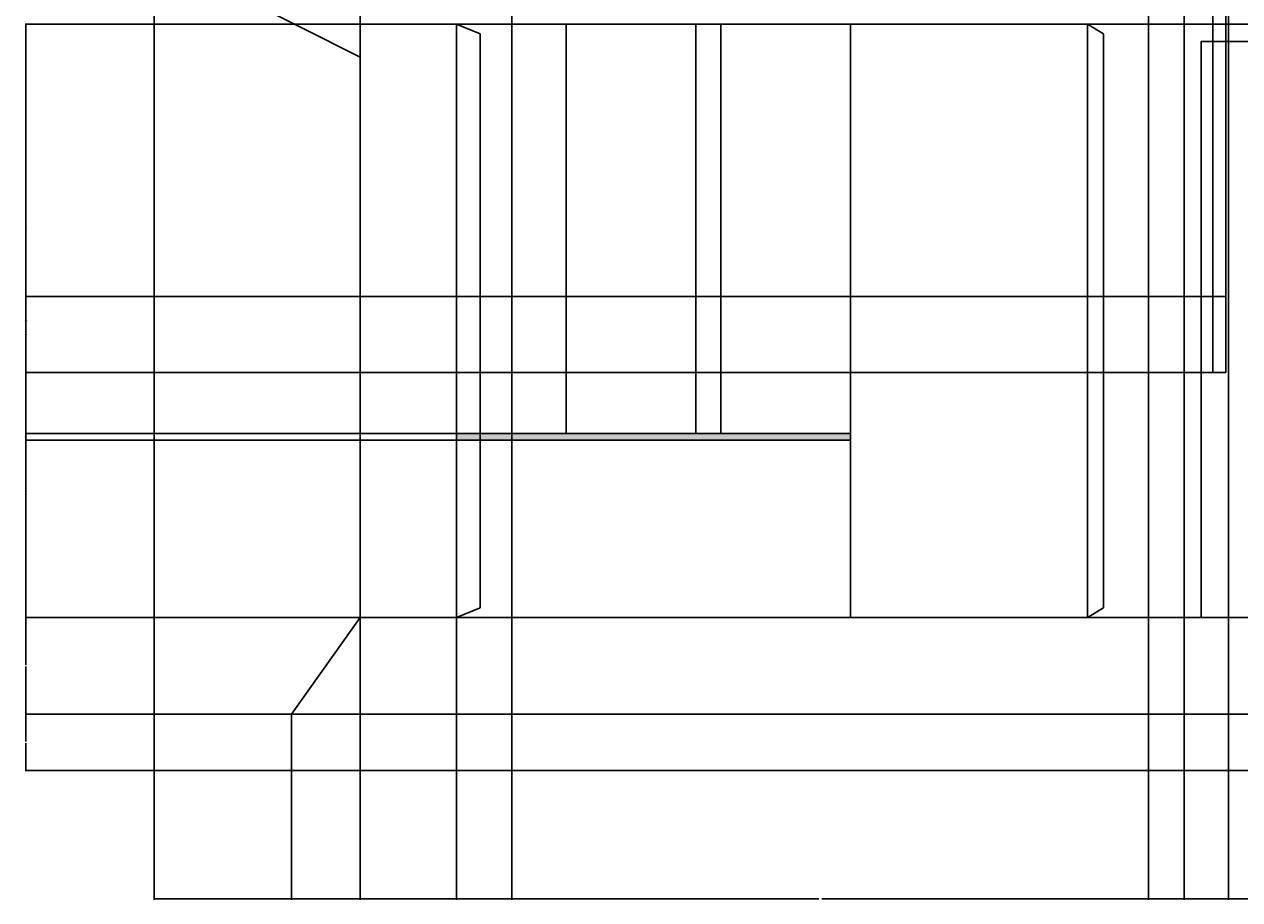
# Model space of a CAD drawing. Units: millimetres. Extents: x 171 to 1599, y 973 to 1509.
# Tile 2 of 7: x 951 to 1235, y 973 to 1178. Entities that reach past the tile are written whole.
import ezdxf

# ---------------------------------------------------------------- set-up
doc = ezdxf.new("R2010")
doc.units = ezdxf.units.MM
for name, color, linetype, lineweight in [('A-ANNO-DIMS', 2, 'Continuous', 18), ('A-ELEV', 7, 'Continuous', 25), ('A-ELEV-FILL', 252, 'Continuous', 13)]:
    doc.layers.add(name, color=color, linetype=linetype, lineweight=lineweight)
doc.styles.get("Standard").update_dxf_attribs({"font": 'arial.ttf'})
doc.dimstyles.get("Standard").update_dxf_attribs({"dimtxt": 0.18, "dimasz": 0.18, "dimexe": 0.18, "dimexo": 0.0625, "dimgap": 0.09, "dimtad": 0, "dimtih": 1, "dimtoh": 1, "dimdec": 1, "dimzin": 0, "dimdsep": 46, "dimlunit": 3, "dimtxsty": 'Standard', "dimcen": 0.09, "dimadec": 0, "dimazin": 0, "dimtfac": 1, "dimtdec": 1, "dimtofl": 0, "dimtmove": 0, "dimatfit": 3, "dimfxl": 1, "dimtolj": 1, "dimtzin": 0, "dimarcsym": 0})

# ---------------------------------------------------------------- blocks, each defined once
blk = doc.blocks.new('*D2')
at = {"layer": 'A-ANNO-DIMS', "color": 0, "lineweight": -2, "transparency": 16777216}
for p, q in [((1043.70287, 1478.130098), (1599.212656, 1478.130098)), ((1599.032656, 1477.950098), (1599.032656, 1240.959874)), ((1599.032656, 1003.60965), (1599.032656, 1240.599874)), ((1348.449149, 1003.42965), (1599.212656, 1003.42965))]:
    blk.add_line(p, q, dxfattribs=at)
at = {"layer": 'A-ANNO-DIMS', "color": 0, "transparency": 16777216}
for points in [[(1599.002656, 1477.950098), (1599.062656, 1477.950098), (1599.032656, 1478.130098)], [(1599.002656, 1003.60965), (1599.062656, 1003.60965), (1599.032656, 1003.42965)]]:
    blk.add_solid(points, dxfattribs=at)
at = {"layer": 'Defpoints', "color": 0, "transparency": 16777216}
for p in [(1043.64037, 1478.130098), (1599.032656, 1478.130098), (1348.386649, 1003.42965)]:
    blk.add_point(p, dxfattribs=at)
at = {"layer": 'A-ANNO-DIMS', "color": 0, "transparency": 16777216, "insert": (1599.032656, 1240.779874), "char_height": 0.18, "attachment_point": 5}
blk.add_mtext('\\A1;474.7', dxfattribs=at)
blk = doc.blocks.new('*D3')
at = {"layer": 'A-ANNO-DIMS', "color": 0, "lineweight": -2, "transparency": 16777216}
for p, q in [((1029.07, 1039.19), (1029.07, 973.25)), ((1013.06, 1003.37), (1013.06, 973.25)), ((1013.24, 973.43), (1020.69, 973.43)), ((1028.89, 973.43), (1021.43, 973.43))]:
    blk.add_line(p, q, dxfattribs=at)
at = {"layer": 'A-ANNO-DIMS', "color": 0, "transparency": 16777216}
for points in [[(1013.24, 973.46), (1013.24, 973.4), (1013.06, 973.43)], [(1028.89, 973.46), (1028.89, 973.4), (1029.07, 973.43)]]:
    blk.add_solid(points, dxfattribs=at)
at = {"layer": 'Defpoints', "color": 0, "transparency": 16777216}
for p in [(1029.07, 1039.25), (1013.06, 1003.43), (1029.07, 973.43)]:
    blk.add_point(p, dxfattribs=at)
at = {"layer": 'A-ANNO-DIMS', "color": 0, "transparency": 16777216, "insert": (1021.06, 973.43), "char_height": 0.18, "attachment_point": 5}
blk.add_mtext('\\A1;16.01', dxfattribs=at)
blk = doc.blocks.new('*D4')
at = {"layer": 'A-ANNO-DIMS', "color": 0, "lineweight": -2, "transparency": 16777216}
for p, q in [((1029.07, 1039.19), (1029.07, 973.25)), ((1051.62, 1039.19), (1051.62, 973.25)), ((1029.25, 973.43), (1039.88, 973.43)), ((1051.44, 973.43), (1040.81, 973.43))]:
    blk.add_line(p, q, dxfattribs=at)
at = {"layer": 'A-ANNO-DIMS', "color": 0, "transparency": 16777216}
for points in [[(1029.25, 973.46), (1029.25, 973.4), (1029.07, 973.43)], [(1051.44, 973.46), (1051.44, 973.4), (1051.62, 973.43)]]:
    blk.add_solid(points, dxfattribs=at)
at = {"layer": 'Defpoints', "color": 0, "transparency": 16777216}
for p in [(1029.07, 1039.25), (1051.62, 1039.25), (1051.62, 973.43)]:
    blk.add_point(p, dxfattribs=at)
at = {"layer": 'A-ANNO-DIMS', "color": 0, "transparency": 16777216, "insert": (1040.34, 973.43), "char_height": 0.18, "attachment_point": 5}
blk.add_mtext('\\A1;22.556', dxfattribs=at)
blk = doc.blocks.new('*D5')
at = {"layer": 'A-ANNO-DIMS', "color": 0, "lineweight": -2, "transparency": 16777216}
for p, q in [((1051.62, 1039.19), (1051.62, 973.25)), ((1221.72, 1039.19), (1221.72, 973.25)), ((1051.8, 973.43), (1136.3, 973.43)), ((1221.54, 973.43), (1137.04, 973.43))]:
    blk.add_line(p, q, dxfattribs=at)
at = {"layer": 'A-ANNO-DIMS', "color": 0, "transparency": 16777216}
for points in [[(1051.8, 973.46), (1051.8, 973.4), (1051.62, 973.43)], [(1221.54, 973.46), (1221.54, 973.4), (1221.72, 973.43)]]:
    blk.add_solid(points, dxfattribs=at)
at = {"layer": 'Defpoints', "color": 0, "transparency": 16777216}
for p in [(1051.62, 1039.25), (1221.72, 1039.25), (1221.72, 973.43)]:
    blk.add_point(p, dxfattribs=at)
at = {"layer": 'A-ANNO-DIMS', "color": 0, "transparency": 16777216, "insert": (1136.67, 973.43), "char_height": 0.18, "attachment_point": 5}
blk.add_mtext('\\A1;170.1', dxfattribs=at)
blk = doc.blocks.new('*D6')
at = {"layer": 'A-ANNO-DIMS', "color": 0, "lineweight": -2, "transparency": 16777216}
for p, q in [((1221.72, 1039.19), (1221.72, 973.25)), ((1298.24, 1039.19), (1298.24, 973.25)), ((1221.9, 973.43), (1259.59, 973.43)), ((1298.06, 973.43), (1260.37, 973.43))]:
    blk.add_line(p, q, dxfattribs=at)
at = {"layer": 'A-ANNO-DIMS', "color": 0, "transparency": 16777216}
for points in [[(1221.9, 973.46), (1221.9, 973.4), (1221.72, 973.43)], [(1298.06, 973.46), (1298.06, 973.4), (1298.24, 973.43)]]:
    blk.add_solid(points, dxfattribs=at)
at = {"layer": 'Defpoints', "color": 0, "transparency": 16777216}
for p in [(1221.72, 1039.25), (1298.24, 1039.25), (1298.24, 973.43)]:
    blk.add_point(p, dxfattribs=at)
at = {"layer": 'A-ANNO-DIMS', "color": 0, "transparency": 16777216, "insert": (1259.98, 973.43), "char_height": 0.18, "attachment_point": 5}
blk.add_mtext('\\A1;76.52', dxfattribs=at)
blk = doc.blocks.new('*D11')
at = {"layer": 'A-ANNO-DIMS', "color": 0, "lineweight": -2, "transparency": 16777216}
for p, q in [((1012.99, 1016.64), (950.75, 1016.64)), ((950.93, 1016.46), (950.93, 1010.22)), ((950.93, 1003.61), (950.93, 1009.85)), ((1012.99, 1003.43), (950.75, 1003.43))]:
    blk.add_line(p, q, dxfattribs=at)
at = {"layer": 'A-ANNO-DIMS', "color": 0, "transparency": 16777216}
for points in [[(950.9, 1016.46), (950.96, 1016.46), (950.93, 1016.64)], [(950.9, 1003.61), (950.96, 1003.61), (950.93, 1003.43)]]:
    blk.add_solid(points, dxfattribs=at)
at = {"layer": 'Defpoints', "color": 0, "transparency": 16777216}
for p in [(950.93, 1016.64), (1013.06, 1016.64), (1013.06, 1003.43)]:
    blk.add_point(p, dxfattribs=at)
at = {"layer": 'A-ANNO-DIMS', "color": 0, "transparency": 16777216, "insert": (950.93, 1010.03), "char_height": 0.18, "attachment_point": 5}
blk.add_mtext('\\A1;13.21', dxfattribs=at)
blk = doc.blocks.new('*D12')
at = {"layer": 'A-ANNO-DIMS', "color": 0, "lineweight": -2, "transparency": 16777216}
for p, q in [((1029, 1039.25), (950.75, 1039.25)), ((950.93, 1039.07), (950.93, 1028.13)), ((950.93, 1016.82), (950.93, 1027.76)), ((1012.99, 1016.64), (950.75, 1016.64))]:
    blk.add_line(p, q, dxfattribs=at)
at = {"layer": 'A-ANNO-DIMS', "color": 0, "transparency": 16777216}
for points in [[(950.9, 1039.07), (950.96, 1039.07), (950.93, 1039.25)], [(950.9, 1016.82), (950.96, 1016.82), (950.93, 1016.64)]]:
    blk.add_solid(points, dxfattribs=at)
at = {"layer": 'Defpoints', "color": 0, "transparency": 16777216}
for p in [(950.93, 1039.25), (1029.07, 1039.25), (1013.06, 1016.64)]:
    blk.add_point(p, dxfattribs=at)
at = {"layer": 'A-ANNO-DIMS', "color": 0, "transparency": 16777216, "insert": (950.93, 1027.94), "char_height": 0.18, "attachment_point": 5}
blk.add_mtext('\\A1;22.61', dxfattribs=at)
blk = doc.blocks.new('*D13')
at = {"layer": 'A-ANNO-DIMS', "color": 0, "lineweight": -2, "transparency": 16777216}
for p, q in [((1029, 1177.87), (950.75, 1177.87)), ((950.93, 1177.69), (950.93, 1108.74)), ((950.93, 1039.43), (950.93, 1108.38)), ((1029, 1039.25), (950.75, 1039.25))]:
    blk.add_line(p, q, dxfattribs=at)
at = {"layer": 'A-ANNO-DIMS', "color": 0, "transparency": 16777216}
for points in [[(950.9, 1177.69), (950.96, 1177.69), (950.93, 1177.87)], [(950.9, 1039.43), (950.96, 1039.43), (950.93, 1039.25)]]:
    blk.add_solid(points, dxfattribs=at)
at = {"layer": 'Defpoints', "color": 0, "transparency": 16777216}
for p in [(950.93, 1177.87), (1029.07, 1177.87), (1029.07, 1039.25)]:
    blk.add_point(p, dxfattribs=at)
at = {"layer": 'A-ANNO-DIMS', "color": 0, "transparency": 16777216, "insert": (950.93, 1108.56), "char_height": 0.18, "attachment_point": 5}
blk.add_mtext('\\A1;138.62', dxfattribs=at)
blk = doc.blocks.new('*D52')
at = {"layer": 'A-ANNO-DIMS', "color": 0, "lineweight": -2, "transparency": 16777216}
for p, q in [((1064.5, 1203.73), (1064.5, 973.25)), ((980.93, 1194.43), (980.93, 973.25)), ((981.11, 973.43), (1022.32, 973.43)), ((1064.32, 973.43), (1023.11, 973.43))]:
    blk.add_line(p, q, dxfattribs=at)
at = {"layer": 'A-ANNO-DIMS', "color": 0, "transparency": 16777216}
for points in [[(981.11, 973.46), (981.11, 973.4), (980.93, 973.43)], [(1064.32, 973.46), (1064.32, 973.4), (1064.5, 973.43)]]:
    blk.add_solid(points, dxfattribs=at)
at = {"layer": 'Defpoints', "color": 0, "transparency": 16777216}
for p in [(1064.5, 1203.79), (980.93, 1194.49), (1064.5, 973.43)]:
    blk.add_point(p, dxfattribs=at)
at = {"layer": 'A-ANNO-DIMS', "color": 0, "transparency": 16777216, "insert": (1022.72, 973.43), "char_height": 0.18, "attachment_point": 5}
blk.add_mtext('\\A1;83.57', dxfattribs=at)
blk = doc.blocks.new('*D53')
at = {"layer": 'A-ANNO-DIMS', "color": 0, "lineweight": -2, "transparency": 16777216}
for p, q in [((1213.35, 1203.73), (1213.35, 973.25)), ((1232.1, 1203.73), (1232.1, 973.25)), ((1213.53, 973.43), (1222.34, 973.43)), ((1231.92, 973.43), (1223.11, 973.43))]:
    blk.add_line(p, q, dxfattribs=at)
at = {"layer": 'A-ANNO-DIMS', "color": 0, "transparency": 16777216}
for points in [[(1213.53, 973.46), (1213.53, 973.4), (1213.35, 973.43)], [(1231.92, 973.46), (1231.92, 973.4), (1232.1, 973.43)]]:
    blk.add_solid(points, dxfattribs=at)
at = {"layer": 'Defpoints', "color": 0, "transparency": 16777216}
for p in [(1213.35, 1203.79), (1232.1, 1203.79), (1232.1, 973.43)]:
    blk.add_point(p, dxfattribs=at)
at = {"layer": 'A-ANNO-DIMS', "color": 0, "transparency": 16777216, "insert": (1222.72, 973.43), "char_height": 0.18, "attachment_point": 5}
blk.add_mtext('\\A1;18.75', dxfattribs=at)
blk = doc.blocks.new('*D54')
at = {"layer": 'A-ANNO-DIMS', "color": 0, "lineweight": -2, "transparency": 16777216}
for p, q in [((1232.1, 1203.73), (1232.1, 973.25)), ((1320.32, 1192.2), (1320.32, 973.25)), ((1232.28, 973.43), (1275.82, 973.43)), ((1320.14, 973.43), (1276.6, 973.43))]:
    blk.add_line(p, q, dxfattribs=at)
at = {"layer": 'A-ANNO-DIMS', "color": 0, "transparency": 16777216}
for points in [[(1232.28, 973.46), (1232.28, 973.4), (1232.1, 973.43)], [(1320.14, 973.46), (1320.14, 973.4), (1320.32, 973.43)]]:
    blk.add_solid(points, dxfattribs=at)
at = {"layer": 'Defpoints', "color": 0, "transparency": 16777216}
for p in [(1232.1, 1203.79), (1320.32, 1192.27), (1320.32, 973.43)]:
    blk.add_point(p, dxfattribs=at)
at = {"layer": 'A-ANNO-DIMS', "color": 0, "transparency": 16777216, "insert": (1276.21, 973.43), "char_height": 0.18, "attachment_point": 5}
blk.add_mtext('\\A1;88.22', dxfattribs=at)
blk = doc.blocks.new('*D71')
at = {"layer": 'A-ANNO-DIMS', "color": 0, "lineweight": -2, "transparency": 16777216}
for p, q in [((1221.72, 1177.93), (1221.72, 1508.31)), ((1221.9, 1508.13), (1224.73, 1508.13)), ((1228.22, 1508.13), (1225.38, 1508.13)), ((1228.4, 1114.32), (1228.4, 1508.31))]:
    blk.add_line(p, q, dxfattribs=at)
at = {"layer": 'A-ANNO-DIMS', "color": 0, "transparency": 16777216}
for points in [[(1221.9, 1508.16), (1221.9, 1508.1), (1221.72, 1508.13)], [(1228.22, 1508.16), (1228.22, 1508.1), (1228.4, 1508.13)]]:
    blk.add_solid(points, dxfattribs=at)
at = {"layer": 'Defpoints', "color": 0, "transparency": 16777216}
for p in [(1228.4, 1508.13), (1221.72, 1177.87), (1228.4, 1114.25)]:
    blk.add_point(p, dxfattribs=at)
at = {"layer": 'A-ANNO-DIMS', "color": 0, "transparency": 16777216, "insert": (1225.06, 1508.13), "char_height": 0.18, "attachment_point": 5}
blk.add_mtext('\\A1;6.68', dxfattribs=at)
blk = doc.blocks.new('*D72')
at = {"layer": 'A-ANNO-DIMS', "color": 0, "lineweight": -2, "transparency": 16777216}
for p, q in [((1228.4, 1114.32), (1228.4, 1508.31)), ((1228.58, 1508.13), (1229.61, 1508.13)), ((1231.28, 1508.13), (1230.25, 1508.13)), ((1231.46, 1114.32), (1231.46, 1508.31))]:
    blk.add_line(p, q, dxfattribs=at)
at = {"layer": 'A-ANNO-DIMS', "color": 0, "transparency": 16777216}
for points in [[(1228.58, 1508.16), (1228.58, 1508.1), (1228.4, 1508.13)], [(1231.28, 1508.16), (1231.28, 1508.1), (1231.46, 1508.13)]]:
    blk.add_solid(points, dxfattribs=at)
at = {"layer": 'Defpoints', "color": 0, "transparency": 16777216}
for p in [(1231.46, 1508.13), (1228.4, 1114.25), (1231.46, 1114.25)]:
    blk.add_point(p, dxfattribs=at)
at = {"layer": 'A-ANNO-DIMS', "color": 0, "transparency": 16777216, "insert": (1229.93, 1508.13), "char_height": 0.18, "attachment_point": 5}
blk.add_mtext('\\A1;3.06', dxfattribs=at)
blk = doc.blocks.new('*D73')
at = {"layer": 'A-ANNO-DIMS', "color": 0, "lineweight": -2, "transparency": 16777216}
for p, q in [((1231.46, 1114.32), (1231.46, 1508.31)), ((1231.64, 1508.13), (1234.06, 1508.13)), ((1237.13, 1508.13), (1234.71, 1508.13)), ((1237.31, 1162.35), (1237.31, 1508.31))]:
    blk.add_line(p, q, dxfattribs=at)
at = {"layer": 'A-ANNO-DIMS', "color": 0, "transparency": 16777216}
for points in [[(1231.64, 1508.16), (1231.64, 1508.1), (1231.46, 1508.13)], [(1237.13, 1508.16), (1237.13, 1508.1), (1237.31, 1508.13)]]:
    blk.add_solid(points, dxfattribs=at)
at = {"layer": 'Defpoints', "color": 0, "transparency": 16777216}
for p in [(1237.31, 1508.13), (1237.31, 1162.29), (1231.46, 1114.25)]:
    blk.add_point(p, dxfattribs=at)
at = {"layer": 'A-ANNO-DIMS', "color": 0, "transparency": 16777216, "insert": (1234.38, 1508.13), "char_height": 0.18, "attachment_point": 5}
blk.add_mtext('\\A1;5.85', dxfattribs=at)
blk = doc.blocks.new('*D81')
at = {"layer": 'A-ANNO-DIMS', "color": 0, "lineweight": -2, "transparency": 16777216}
for p, q in [((1143.64, 1080.67), (950.75, 1080.67)), ((950.93, 1080.49), (950.93, 1060.14)), ((950.93, 1039.43), (950.93, 1059.78)), ((1143.64, 1039.25), (950.75, 1039.25))]:
    blk.add_line(p, q, dxfattribs=at)
at = {"layer": 'A-ANNO-DIMS', "color": 0, "transparency": 16777216}
for points in [[(950.9, 1080.49), (950.96, 1080.49), (950.93, 1080.67)], [(950.9, 1039.43), (950.96, 1039.43), (950.93, 1039.25)]]:
    blk.add_solid(points, dxfattribs=at)
at = {"layer": 'Defpoints', "color": 0, "transparency": 16777216}
for p in [(950.93, 1080.67), (1143.7, 1080.67), (1143.7, 1039.25)]:
    blk.add_point(p, dxfattribs=at)
at = {"layer": 'A-ANNO-DIMS', "color": 0, "transparency": 16777216, "insert": (950.93, 1059.96), "char_height": 0.18, "attachment_point": 5}
blk.add_mtext('\\A1;41.42', dxfattribs=at)
blk = doc.blocks.new('*D82')
at = {"layer": 'A-ANNO-DIMS', "color": 0, "lineweight": -2, "transparency": 16777216}
for p, q in [((1143.64, 1082.23), (950.75, 1082.23)), ((1143.64, 1080.67), (950.75, 1080.67)), ((950.93, 1082.05), (950.93, 1081.63)), ((950.93, 1080.85), (950.93, 1081.27))]:
    blk.add_line(p, q, dxfattribs=at)
at = {"layer": 'A-ANNO-DIMS', "color": 0, "transparency": 16777216}
for points in [[(950.9, 1082.05), (950.96, 1082.05), (950.93, 1082.23)], [(950.9, 1080.85), (950.96, 1080.85), (950.93, 1080.67)]]:
    blk.add_solid(points, dxfattribs=at)
at = {"layer": 'Defpoints', "color": 0, "transparency": 16777216}
for p in [(950.93, 1082.23), (1143.7, 1082.23), (1143.7, 1080.67)]:
    blk.add_point(p, dxfattribs=at)
at = {"layer": 'A-ANNO-DIMS', "color": 0, "transparency": 16777216, "insert": (950.93, 1081.45), "char_height": 0.18, "attachment_point": 5}
blk.add_mtext('\\A1;1.561', dxfattribs=at)
blk = doc.blocks.new('*D83')
at = {"layer": 'A-ANNO-DIMS', "color": 0, "lineweight": -2, "transparency": 16777216}
for p, q in [((1143.64, 1177.87), (950.75, 1177.87)), ((950.93, 1177.69), (950.93, 1130.23)), ((950.93, 1082.41), (950.93, 1129.87)), ((1143.64, 1082.23), (950.75, 1082.23))]:
    blk.add_line(p, q, dxfattribs=at)
at = {"layer": 'A-ANNO-DIMS', "color": 0, "transparency": 16777216}
for points in [[(950.9, 1177.69), (950.96, 1177.69), (950.93, 1177.87)], [(950.9, 1082.41), (950.96, 1082.41), (950.93, 1082.23)]]:
    blk.add_solid(points, dxfattribs=at)
at = {"layer": 'Defpoints', "color": 0, "transparency": 16777216}
for p in [(950.93, 1177.87), (1143.7, 1177.87), (1143.7, 1082.23)]:
    blk.add_point(p, dxfattribs=at)
at = {"layer": 'A-ANNO-DIMS', "color": 0, "transparency": 16777216, "insert": (950.93, 1130.05), "char_height": 0.18, "attachment_point": 5}
blk.add_mtext('\\A1;95.64', dxfattribs=at)
blk = doc.blocks.new('*D84')
at = {"layer": 'A-ANNO-DIMS', "color": 0, "lineweight": -2, "transparency": 16777216}
for p, q in [((1228.34, 1096.49), (950.75, 1096.49)), ((950.93, 1096.31), (950.93, 1068.05)), ((950.93, 1039.43), (950.93, 1067.69)), ((1221.66, 1039.25), (950.75, 1039.25))]:
    blk.add_line(p, q, dxfattribs=at)
at = {"layer": 'A-ANNO-DIMS', "color": 0, "transparency": 16777216}
for points in [[(950.9, 1096.31), (950.96, 1096.31), (950.93, 1096.49)], [(950.9, 1039.43), (950.96, 1039.43), (950.93, 1039.25)]]:
    blk.add_solid(points, dxfattribs=at)
at = {"layer": 'Defpoints', "color": 0, "transparency": 16777216}
for p in [(950.93, 1096.49), (1228.4, 1096.49), (1221.72, 1039.25)]:
    blk.add_point(p, dxfattribs=at)
at = {"layer": 'A-ANNO-DIMS', "color": 0, "transparency": 16777216, "insert": (950.93, 1067.87), "char_height": 0.18, "attachment_point": 5}
blk.add_mtext('\\A1;57.25', dxfattribs=at)
blk = doc.blocks.new('*D85')
at = {"layer": 'A-ANNO-DIMS', "color": 0, "lineweight": -2, "transparency": 16777216}
for p, q in [((1228.34, 1114.25), (950.75, 1114.25)), ((950.93, 1114.07), (950.93, 1105.56)), ((950.93, 1096.67), (950.93, 1105.19)), ((1228.34, 1096.49), (950.75, 1096.49))]:
    blk.add_line(p, q, dxfattribs=at)
at = {"layer": 'A-ANNO-DIMS', "color": 0, "transparency": 16777216}
for points in [[(950.9, 1114.07), (950.96, 1114.07), (950.93, 1114.25)], [(950.9, 1096.67), (950.96, 1096.67), (950.93, 1096.49)]]:
    blk.add_solid(points, dxfattribs=at)
at = {"layer": 'Defpoints', "color": 0, "transparency": 16777216}
for p in [(950.93, 1114.25), (1228.4, 1114.25), (1228.4, 1096.49)]:
    blk.add_point(p, dxfattribs=at)
at = {"layer": 'A-ANNO-DIMS', "color": 0, "transparency": 16777216, "insert": (950.93, 1105.37), "char_height": 0.18, "attachment_point": 5}
blk.add_mtext('\\A1;17.76', dxfattribs=at)

msp = doc.modelspace()

# ---------------------------------------------------------------- hatches: boundary and pattern name
at = {"layer": 'A-ELEV-FILL'}
h = msp.add_hatch(color=256, dxfattribs=at)
h.dxf.hatch_style = 1
h.paths.add_polyline_path([(1057.1375, 1082.2327), (1051.6226, 1082.2327), (1051.6226, 1080.6718), (1057.1375, 1080.6718)])
h.paths.add_polyline_path([(1143.7, 1082.2327), (1057.1375, 1082.2327), (1057.1375, 1080.6718), (1143.7, 1080.6718)])
h.paths.add_polyline_path([(1509.9876, 1082.2327), (1504.7689, 1082.2327), (1504.7689, 1080.6718), (1509.0669, 1080.6718), (1509.9876, 1080.6718)])
h.paths.add_polyline_path([(1443.1972, 1082.2327), (1328.4737, 1082.2327), (1328.4737, 1080.6718), (1329.4402, 1080.6718), (1443.1972, 1080.6718)])

# ---------------------------------------------------------------- linework, layer by layer
at = {"layer": 'A-ELEV'}
for p, q in [((1029.0669, 1170.1702), (980.9303, 1194.488)), ((1029.0669, 1177.8722), (1029.0669, 1181.6916)), ((1064.505, 1177.8722), (1029.0669, 1177.8722)), ((1051.6226, 1177.8722), (1057.1375, 1175.6512)), ((1064.505, 1082.2327), (1064.505, 1177.8722)), ((1064.505, 1177.8722), (1077.2721, 1177.8722)), ((1077.2721, 1177.8722), (1077.2721, 1082.2327)), ((1199.109, 1177.8722), (1202.8388, 1175.6512)), ((1057.1375, 1175.6512), (1057.1375, 1041.4702)), ((1202.8388, 1175.6512), (1202.8388, 1041.4702)), ((1029.0669, 1146.0387), (1029.0669, 1152.0387)), ((1051.6226, 1039.2493), (1057.1375, 1041.4702)), ((1199.109, 1039.2493), (1202.8388, 1041.4702)), ((1013.0567, 1003.4297), (1013.0567, 1016.6402))]:
    msp.add_line(p, q, dxfattribs=at)
for points in [[(1064.505, 1177.8722), (1298.2363, 1177.8722), (1298.2363, 1181.6916), (1064.505, 1181.6916)], [(1225.7194, 1039.2493), (1225.7194, 1173.8722), (1294.2363, 1173.8722), (1294.2363, 1039.2493)], [(1143.7, 1039.2493), (1143.7, 1080.6718), (1051.6226, 1080.6718), (1051.6226, 1039.2493)], [(1329.4402, 1039.2493), (1348.3866, 1016.6402), (1013.0567, 1016.6402), (1029.0669, 1039.2493)], [(1029.0669, 1039.2493), (1329.4402, 1039.2493)], [(1348.3866, 1003.4297), (1013.0567, 1003.4297)]]:
    msp.add_lwpolyline(points, dxfattribs=at)
for points in [[(1029.0669, 1177.8722), (1051.6226, 1177.8722), (1051.6226, 1039.2493), (1029.0669, 1039.2493)], [(1107.5629, 1177.8722), (1113.4097, 1177.8722), (1113.4097, 1082.2327), (1107.5629, 1082.2327)], [(1143.7, 1177.8722), (1199.109, 1177.8722), (1199.109, 1039.2493), (1143.7, 1039.2493)], [(1298.2363, 1039.2493), (1221.7194, 1039.2493), (1221.7194, 1177.8722), (1298.2363, 1177.8722)], [(1231.4586, 1096.495), (1228.3992, 1096.495), (1228.3992, 1114.2546), (1231.4586, 1114.2546)], [(1143.7, 1080.6718), (1051.6226, 1080.6718), (1051.6226, 1082.2327), (1143.7, 1082.2327)]]:
    msp.add_lwpolyline(points, close=True, dxfattribs=at)

# ---------------------------------------------------------------- dimensions: what is measured, and where the dimension line sits
at = {"layer": 'A-ANNO-DIMS'}
for base, p1, p2, override, picture, middle in [((1228.3992, 1508.1301), (1221.7194, 1177.8722), (1228.3992, 1114.2546), {"dimdec": 2, "dimlfac": 1, "dimrnd": 0, "dimzin": 0, "dimdsep": 46, "dimlunit": 2}, '*D71', (1225.0593, 1508.1301)), ((1231.4586, 1508.1301), (1228.3992, 1114.2546), (1231.4586, 1114.2546), {"dimdec": 2, "dimlfac": 1, "dimrnd": 0, "dimzin": 0, "dimdsep": 46, "dimlunit": 2}, '*D72', (1229.9289, 1508.1301)), ((1237.3083, 1508.1301), (1231.4586, 1114.2546), (1237.3083, 1162.2854), {"dimdec": 2, "dimlfac": 1, "dimrnd": 0, "dimzin": 0, "dimdsep": 46, "dimlunit": 2}, '*D73', (1234.3834, 1508.1301)), ((1064.505, 973.4297), (980.9303, 1194.488), (1064.505, 1203.7941), {"dimdec": 2, "dimlfac": 1, "dimrnd": 0, "dimzin": 0, "dimdsep": 46, "dimlunit": 2}, '*D52', (1022.7176, 973.4297)), ((1232.0993, 973.4297), (1213.3488, 1203.7941), (1232.0993, 1203.7941), {"dimdec": 2, "dimlfac": 1, "dimrnd": 0, "dimzin": 0, "dimdsep": 46, "dimlunit": 2}, '*D53', (1222.724, 973.4297)), ((1320.3201, 973.4297), (1232.0993, 1203.7941), (1320.3201, 1192.267), {"dimdec": 2, "dimlfac": 1, "dimrnd": 0, "dimzin": 0, "dimdsep": 46, "dimlunit": 2}, '*D54', (1276.2097, 973.4297)), ((1029.0669, 973.4297), (1013.0567, 1003.4297), (1029.0669, 1039.2493), {"dimdec": 2, "dimlfac": 1, "dimrnd": 0, "dimzin": 0, "dimdsep": 46, "dimlunit": 2}, '*D3', (1021.0618, 973.4297)), ((1051.6226, 973.4297), (1029.0669, 1039.2493), (1051.6226, 1039.2493), {"dimdec": 3, "dimlfac": 1, "dimrnd": 0, "dimzin": 0, "dimdsep": 46, "dimlunit": 2}, '*D4', (1040.3447, 973.4297)), ((1221.7194, 973.4297), (1051.6226, 1039.2493), (1221.7194, 1039.2493), {"dimdec": 1, "dimlfac": 1, "dimrnd": 0, "dimzin": 0, "dimdsep": 46, "dimlunit": 2}, '*D5', (1136.671, 973.4297)), ((1298.2363, 973.4297), (1221.7194, 1039.2493), (1298.2363, 1039.2493), {"dimdec": 2, "dimlfac": 1, "dimrnd": 0, "dimzin": 0, "dimdsep": 46, "dimlunit": 2}, '*D6', (1259.9779, 973.4297))]:
    dim = msp.add_linear_dim(base=base, p1=p1, p2=p2, dimstyle='Standard', override=override, dxfattribs=at)
    dim.commit()
    dim.dimension.update_dxf_attribs({"geometry": picture, "text_midpoint": middle})
for base, p1, p2, override, picture, middle in [((1599.0327, 1478.1301), (1348.3866, 1003.4297), (1043.6404, 1478.1301), {"dimdec": 1, "dimlfac": 1, "dimrnd": 0, "dimzin": 0, "dimdsep": 46, "dimlunit": 2}, '*D2', (1599.0327, 1240.7799)), ((950.9303, 1177.8722), (1029.0669, 1039.2493), (1029.0669, 1177.8722), {"dimdec": 2, "dimlfac": 1, "dimrnd": 0, "dimzin": 0, "dimdsep": 46, "dimlunit": 2}, '*D13', (950.9303, 1108.5607)), ((950.9303, 1177.8722), (1143.7, 1082.2327), (1143.7, 1177.8722), {"dimdec": 2, "dimlfac": 1, "dimrnd": 0, "dimzin": 0, "dimdsep": 46, "dimlunit": 2}, '*D83', (950.9303, 1130.0525)), ((950.9303, 1114.2546), (1228.3992, 1096.495), (1228.3992, 1114.2546), {"dimdec": 2, "dimlfac": 1, "dimrnd": 0, "dimzin": 0, "dimdsep": 46, "dimlunit": 2}, '*D85', (950.9303, 1105.3748)), ((950.9303, 1096.495), (1221.7194, 1039.2493), (1228.3992, 1096.495), {"dimdec": 2, "dimlfac": 1, "dimrnd": 0, "dimzin": 0, "dimdsep": 46, "dimlunit": 2}, '*D84', (950.9303, 1067.8721)), ((950.9303, 1082.2327), (1143.7, 1080.6718), (1143.7, 1082.2327), {"dimdec": 3, "dimlfac": 1, "dimrnd": 0, "dimzin": 0, "dimdsep": 46, "dimlunit": 2}, '*D82', (950.9303, 1081.4523)), ((950.9303, 1080.6718), (1143.7, 1039.2493), (1143.7, 1080.6718), {"dimdec": 2, "dimlfac": 1, "dimrnd": 0, "dimzin": 0, "dimdsep": 46, "dimlunit": 2}, '*D81', (950.9303, 1059.9606)), ((950.9303, 1039.2493), (1013.0567, 1016.6402), (1029.0669, 1039.2493), {"dimdec": 2, "dimlfac": 1, "dimrnd": 0, "dimzin": 0, "dimdsep": 46, "dimlunit": 2}, '*D12', (950.9303, 1027.9447)), ((950.9303, 1016.6402), (1013.0567, 1003.4297), (1013.0567, 1016.6402), {"dimdec": 2, "dimlfac": 1, "dimrnd": 0, "dimzin": 0, "dimdsep": 46, "dimlunit": 2}, '*D11', (950.9303, 1010.0349))]:
    dim = msp.add_linear_dim(base=base, p1=p1, p2=p2, angle=90, dimstyle='Standard', override=override, dxfattribs=at)
    dim.commit()
    dim.dimension.update_dxf_attribs({"geometry": picture, "text_midpoint": middle})

doc.saveas('drawing.dxf')
